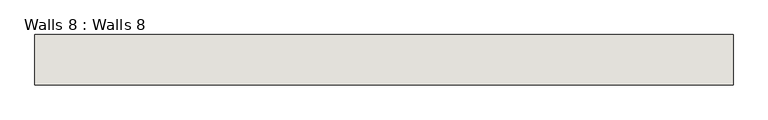
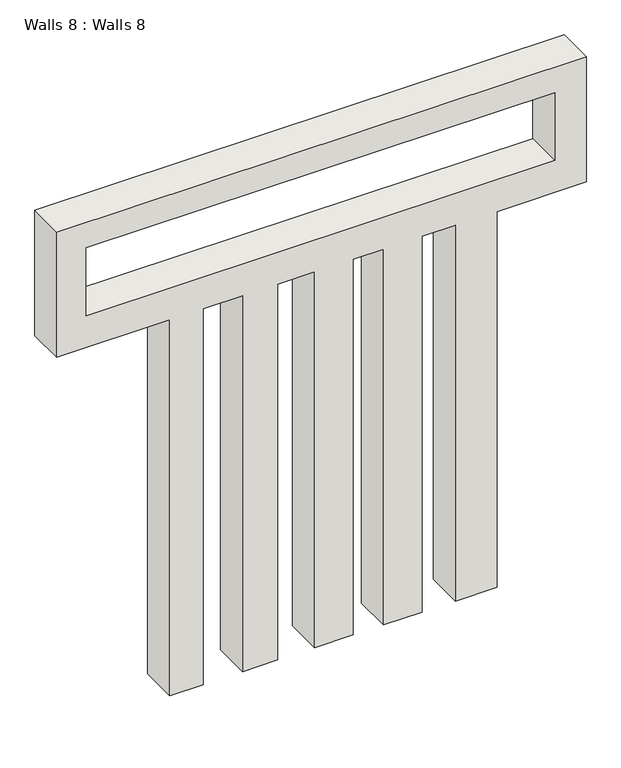
"""IFC4 building model written with IfcOpenShell, lengths in millimetres: wall geometry, Walls 8 : Walls 8."""

from ifc_helpers import new_model, si_unit, frame, origin, place, context, project, spatial, polyline, outline, extrude, source, transform, mapped, element, save


def walls_8_walls_8_a9e6a938(model_context):
    return source(origin(), model_context, "Body", "SweptSolid", [
        extrude(outline(polyline([(7620.0, -6106.9483213), (7620.0, -5954.5483213), (9448.8, -5954.5483213), (9448.8, -5772.2766957), (7620.0, -5772.2766957), (7620.0, -5610.0665483), (9448.8, -5610.0665483), (9448.8, -5440.4832124), (7620.0, -5440.4832124), (7620.0, -5263.526688), (9448.8, -5263.526688), (9448.8, -5122.8311901), (7620.0, -5122.8311901), (7620.0, -4944.6813589), (9448.8, -4944.6813589), (9448.8, -4791.6426228), (7620.0, -4791.6426228), (7620.0, -4599.9397213), (9448.8, -4599.9397213), (9448.8, -4189.1665638), (10058.4, -4189.1665638), (10058.4, -6627.5665638), (9448.8, -6627.5665638), (9448.8, -6106.9483213), (7620.0, -6106.9483213)]), holes=[polyline([(9934.4672706, -4333.5166808), (9604.2672706, -4333.5166808), (9604.2672706, -6492.5166808), (9934.4672706, -6492.5166808), (9934.4672706, -4333.5166808)])]), frame((0.0, -4421.0848411, 0.0), z_axis=(0.0, 1.0, 0.0), x_axis=(0.0, 0.0, 1.0)), (0.0, 0.0, 1.0), 175.3708899),
    ])


if __name__ == "__main__":
    model = new_model("IFC4")
    model_context = context("Model", 3, world=origin())
    ifc_project = project(units=[si_unit("LENGTHUNIT", "METRE", prefix="MILLI")], contexts=[model_context])
    site = spatial("IfcSite", under=ifc_project)
    building = spatial("IfcBuilding", under=site)
    placement = place(None, origin())
    walls_8_walls_8_shape = walls_8_walls_8_a9e6a938(model_context)
    element("IfcWall", 1, ObjectType="Walls 8 : Walls 8", at=placement, inside=building, context=model_context, shape_type="MappedRepresentation", body=[
        mapped(walls_8_walls_8_shape, transform((0.0, 0.0, 0.0), x_axis=(1.0, 0.0, 0.0), y_axis=(0.0, 1.0, 0.0), z_axis=(0.0, 0.0, 1.0))),
    ])
    save(model, "model.ifc")

# Revit data of these elements
# Element 1 (IfcWall, "Walls 8 : Walls 8")
#   Materials on its faces: "Default Wall"
# Materials
#   "Default Wall": colour RGB 128 128 128, transparency 0
